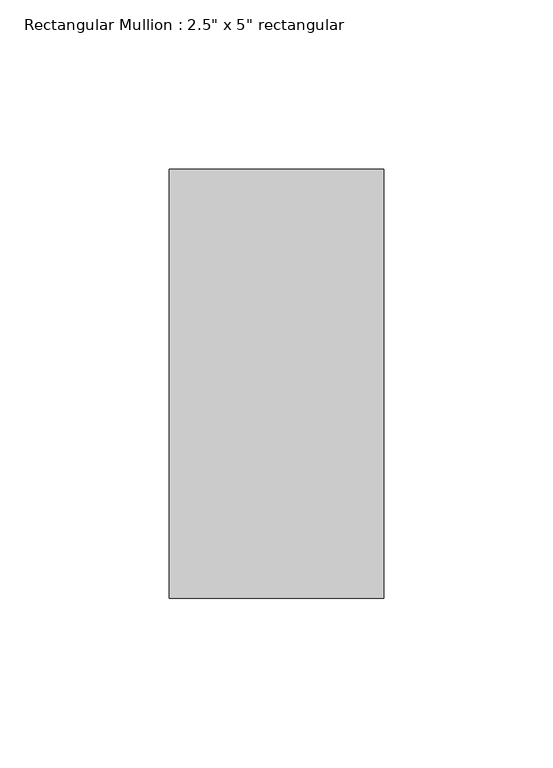
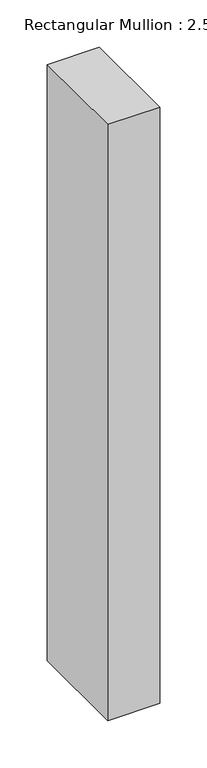
"""IFC4 building model written with IfcOpenShell, lengths in millimetres: member geometry."""

from ifc_helpers import new_model, si_unit, frame, origin, place, context, project, spatial, polyline, outline, extrude, source, transform, mapped, element, save


def member_46f5bc36(model_context):
    return source(origin(), model_context, "Body", "SweptSolid", [
        extrude(outline(polyline([(0.0, 63.5), (0.0, -63.5), (-63.5, -63.5), (-63.5, 63.5), (0.0, 63.5)])), frame((0.0, 0.0, -768.35), z_axis=(0.0, 0.0, 1.0), x_axis=(1.0, 0.0, 0.0)), (0.0, 0.0, 1.0), 768.35),
    ])


if __name__ == "__main__":
    model = new_model("IFC4")
    model_context = context("Model", 3, world=origin())
    ifc_project = project(units=[si_unit("LENGTHUNIT", "METRE", prefix="MILLI")], contexts=[model_context])
    site = spatial("IfcSite", under=ifc_project)
    building = spatial("IfcBuilding", under=site)
    placement = place(None, origin())
    member_shape = member_46f5bc36(model_context)
    element("IfcMember", 1, ObjectType="Rectangular Mullion : 2.5\" x 5\" rectangular", at=placement, inside=building, context=model_context, shape_type="MappedRepresentation", body=[
        mapped(member_shape, transform((0.0, 0.0, 0.0), x_axis=(1.0, 0.0, 0.0), y_axis=(0.0, 1.0, 0.0), z_axis=(0.0, 0.0, 1.0))),
    ])
    save(model, "model.ifc")

# Revit data of these elements
# Type "Rectangular Mullion : 2.5\" x 5\" rectangular"
#   built-in parameter 1007304 = 0.416667 (stored number, unit not read)
#   built-in parameter 1007301 = 0.104167 (stored number, unit not read)
#   built-in parameter 1007300 = 0.104167 (stored number, unit not read)
# Element 1 (IfcMember, "Rectangular Mullion : 2.5\" x 5\" rectangular")
#   Materials on its faces: "Aluminum"
# Materials
#   "Aluminum": class "Metal", colour RGB 247 247 247, transparency 0, Description = "Aluminum 6061", Cost = 0
